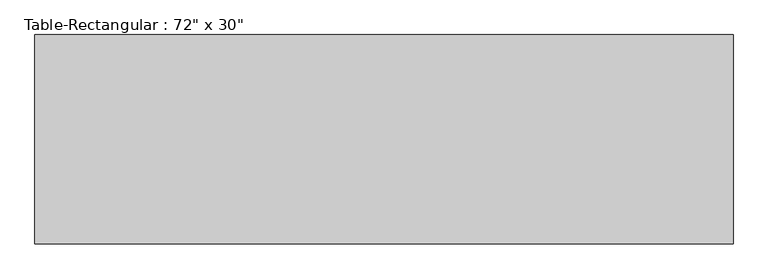
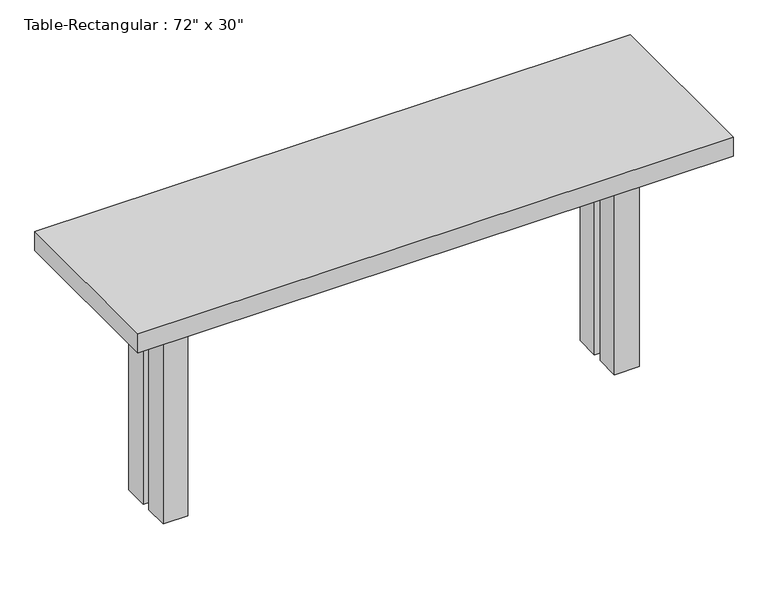
"""IFC4 building model written with IfcOpenShell, lengths in millimetres: furniture geometry."""

from ifc_helpers import new_model, si_unit, frame, origin, origin_with_axes, place, context, project, spatial, polyline, outline, extrude, source, transform, mapped, element, save


def furniture_d94a64e0(model_context):
    return source(origin(), model_context, "Body", "SweptSolid", [
        extrude(outline(polyline([(546.1, 38.1), (546.1, 12.7), (-546.1, 12.7), (-546.1, 38.1), (546.1, 38.1)])), frame((0.0, 0.0, 508.0), z_axis=(0.0, 0.0, 1.0), x_axis=(1.0, 0.0, 0.0)), (0.0, 0.0, 1.0), 101.6),
        extrude(outline(polyline([(546.1, -38.1), (-546.1, -38.1), (-546.1, -12.7), (546.1, -12.7), (546.1, -38.1)])), frame((0.0, 0.0, 508.0), z_axis=(0.0, 0.0, 1.0), x_axis=(1.0, 0.0, 0.0)), (0.0, 0.0, 1.0), 101.6),
        extrude(outline(polyline([(-558.8, -12.7), (-584.2, -12.7), (-584.2, 12.7), (-558.8, 12.7), (-558.8, -12.7)])), frame((0.0, 0.0, 508.0), z_axis=(0.0, 0.0, 1.0), x_axis=(1.0, 0.0, 0.0)), (0.0, 0.0, 1.0), 101.6),
        extrude(outline(polyline([(558.8, -12.7), (558.8, 12.7), (584.2, 12.7), (584.2, -12.7), (558.8, -12.7)])), frame((0.0, 0.0, 508.0), z_axis=(0.0, 0.0, 1.0), x_axis=(1.0, 0.0, 0.0)), (0.0, 0.0, 1.0), 101.6),
        extrude(outline(polyline([(762.0, 228.6), (762.0, -228.6), (-762.0, -228.6), (-762.0, 228.6), (762.0, 228.6)])), frame((0.0, 0.0, 609.6), z_axis=(0.0, 0.0, 1.0), x_axis=(1.0, 0.0, 0.0)), (0.0, 0.0, 1.0), 50.8),
        extrude(outline(polyline([(-546.1, 76.2), (-546.1, 12.7), (-609.6, 12.7), (-609.6, 76.2), (-546.1, 76.2)])), origin_with_axes(), (0.0, 0.0, 1.0), 609.6),
        extrude(outline(polyline([(546.1, 76.2), (609.6, 76.2), (609.6, 12.7), (546.1, 12.7), (546.1, 76.2)])), origin_with_axes(), (0.0, 0.0, 1.0), 609.6),
        extrude(outline(polyline([(-546.1, -76.2), (-609.6, -76.2), (-609.6, -12.7), (-546.1, -12.7), (-546.1, -76.2)])), origin_with_axes(), (0.0, 0.0, 1.0), 609.6),
        extrude(outline(polyline([(546.1, -76.2), (546.1, -12.7), (609.6, -12.7), (609.6, -76.2), (546.1, -76.2)])), origin_with_axes(), (0.0, 0.0, 1.0), 609.6),
    ])


if __name__ == "__main__":
    model = new_model("IFC4")
    model_context = context("Model", 3, world=origin())
    ifc_project = project(units=[si_unit("LENGTHUNIT", "METRE", prefix="MILLI")], contexts=[model_context])
    site = spatial("IfcSite", under=ifc_project)
    building = spatial("IfcBuilding", under=site)
    placement = place(None, origin())
    furniture_shape = furniture_d94a64e0(model_context)
    element("IfcFurniture", 1, ObjectType="Table-Rectangular : 72\" x 30\"", at=placement, inside=building, context=model_context, shape_type="MappedRepresentation", body=[
        mapped(furniture_shape, transform((0.0, 0.0, 0.0), x_axis=(1.0, 0.0, 0.0), y_axis=(0.0, 1.0, 0.0), z_axis=(0.0, 0.0, 1.0))),
    ])
    save(model, "model.ifc")

# Revit data of these elements
# Type "Table-Rectangular : 72\" x 30\""
#   Assembly Code = "E2020200"
#   Height = 2' - 2"
#   Length = 5' - 0"
#   Width = 1' - 6"
#   Base Material = Birch
#   Top Material = Birch
#   Default Elevation = 0
# Element 1 (IfcFurniture, "Table-Rectangular : 72\" x 30\"")
#   Materials on its faces: "Birch"
# Materials
#   "Birch": class "Wood", colour RGB 210 159 95, transparency 0, Description = "Betula Alleghaniensis", Cost = 0
